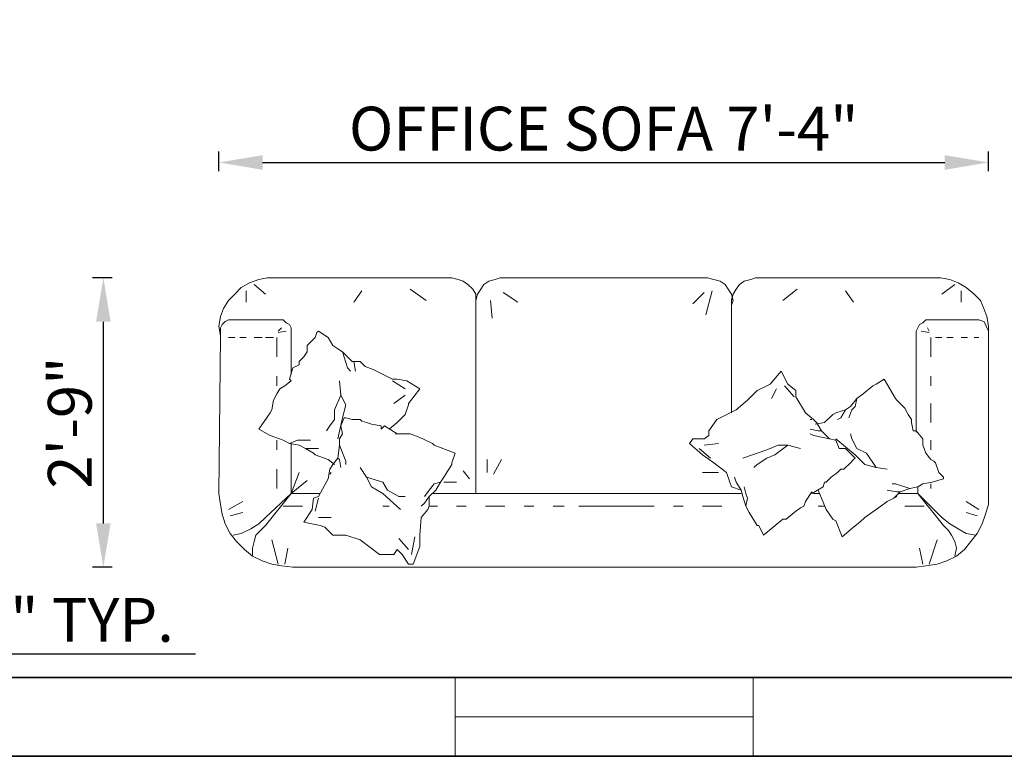
# Model space of a CAD drawing. Units: inches. Extents: x -100 to 766, y -562 to 63.
# Tile 4 of 11: x 268 to 380, y -467 to -383. Entities that reach past the tile are written whole.
import ezdxf

# ---------------------------------------------------------------- set-up
doc = ezdxf.new("R2010")
doc.units = ezdxf.units.IN
for name, color, linetype, lineweight in [('A-ANNO-DIMS', 2, 'Continuous', 18), ('A-GLAZ', 4, 'Continuous', 18), ('A-WALL', 7, 'Continuous', 35), ('furn', 8, 'Continuous', 13)]:
    doc.layers.add(name, color=color, linetype=linetype, lineweight=lineweight)
doc.styles.get("Standard").update_dxf_attribs({"font": 'arial.ttf'})
doc.dimstyles.new('ISO-25', dxfattribs={"dimtxt": 5, "dimasz": 5, "dimexe": 1.25, "dimexo": 0.625, "dimtad": 1, "dimlunit": 3, "dimtxsty": 'Standard', "dimcen": 2.5, "dimadec": 0, "dimazin": 0, "dimtfac": 1, "dimtmove": 0, "dimatfit": 3, "dimfxl": 1, "dimfxlon": 1, "dimarcsym": 0})

# ---------------------------------------------------------------- blocks, each defined once
blk = doc.blocks.new('sofa-36')
at = {"color": 0, "linetype": 'ByBlock'}
for p, q in [((-0.135, 0.885), (-0.105, 0.895)), ((-0.105, 0.895), (-0.135, 0.885)), ((-0.105, 0.895), (-0.08, 0.9)), ((-0.08, 0.9), (-0.105, 0.895)), ((-0.08, 0.9), (0.495, 0.9)), ((0.495, 0.9), (-0.08, 0.9)), ((0.495, 0.9), (0.515, 0.895)), ((0.515, 0.895), (0.495, 0.9)), ((0.515, 0.895), (0.53, 0.89)), ((0.53, 0.89), (0.515, 0.895)), ((0.53, 0.89), (0.545, 0.88)), ((0.545, 0.88), (0.53, 0.89)), ((0.595, 0.88), (0.61, 0.89)), ((0.595, 0.88), (0.61, 0.89)), ((0.61, 0.89), (0.63, 0.895)), ((0.61, 0.89), (0.63, 0.895)), ((0.63, 0.895), (0.645, 0.9)), ((0.63, 0.895), (0.645, 0.9)), ((0.645, 0.9), (0.87, 0.9)), ((0.87, 0.9), (0.645, 0.9)), ((0.87, 0.9), (1.29, 0.9)), ((1.29, 0.9), (0.87, 0.9)), ((1.29, 0.9), (1.31, 0.895)), ((1.31, 0.895), (1.29, 0.9)), ((1.31, 0.895), (1.33, 0.89)), ((1.33, 0.89), (1.31, 0.895)), ((1.33, 0.89), (1.345, 0.88)), ((1.345, 0.88), (1.33, 0.89)), ((1.39, 0.88), (1.405, 0.89)), ((1.39, 0.88), (1.405, 0.89)), ((1.405, 0.89), (1.425, 0.895)), ((1.405, 0.89), (1.425, 0.895)), ((1.425, 0.895), (1.44, 0.9)), ((1.425, 0.895), (1.44, 0.9)), ((1.44, 0.9), (2.015, 0.9)), ((2.015, 0.9), (1.44, 0.9)), ((2.015, 0.9), (2.045, 0.895)), ((2.045, 0.895), (2.015, 0.9)), ((2.045, 0.895), (2.07, 0.885)), ((2.07, 0.885), (2.045, 0.895)), ((-0.18, 0.85), (-0.16, 0.87)), ((-0.16, 0.87), (-0.18, 0.85)), ((-0.16, 0.87), (-0.135, 0.885)), ((-0.135, 0.885), (-0.16, 0.87)), ((-0.145, 0.825), (-0.145, 0.86)), ((-0.085, 0.85), (-0.12, 0.88)), ((0.19, 0.825), (0.215, 0.86)), ((0.415, 0.83), (0.365, 0.865)), ((0.545, 0.88), (0.56, 0.865)), ((0.56, 0.865), (0.545, 0.88)), ((0.56, 0.865), (0.57, 0.85)), ((0.57, 0.85), (0.56, 0.865)), ((0.575, 0.85), (0.585, 0.865)), ((0.575, 0.85), (0.585, 0.865)), ((0.585, 0.865), (0.595, 0.88)), ((0.585, 0.865), (0.595, 0.88)), ((1.305, 0.86), (1.285, 0.785)), ((1.345, 0.88), (1.355, 0.865)), ((1.355, 0.865), (1.345, 0.88)), ((1.355, 0.865), (1.365, 0.85)), ((1.365, 0.85), (1.355, 0.865)), ((1.37, 0.85), (1.38, 0.865)), ((1.37, 0.85), (1.38, 0.865)), ((1.38, 0.865), (1.39, 0.88)), ((1.38, 0.865), (1.39, 0.88)), ((1.525, 0.83), (1.57, 0.865)), ((1.745, 0.825), (1.72, 0.86)), ((2.02, 0.85), (2.06, 0.88)), ((2.07, 0.885), (2.095, 0.87)), ((2.095, 0.87), (2.07, 0.885)), ((2.08, 0.825), (2.08, 0.86)), ((2.095, 0.87), (2.12, 0.85)), ((2.12, 0.85), (2.095, 0.87)), ((-0.215, 0.805), (-0.2, 0.83)), ((-0.2, 0.83), (-0.215, 0.805)), ((-0.2, 0.83), (-0.18, 0.85)), ((-0.18, 0.85), (-0.2, 0.83)), ((0.57, 0.83), (0.575, 0.85)), ((0.57, 0.85), (0.57, 0.83)), ((0.57, 0.83), (0.57, 0.85)), ((0.57, 0.83), (0.575, 0.85)), ((0.57, 0.835), (0.57, 0.23)), ((0.57, 0.815), (0.57, 0.83)), ((0.57, 0.815), (0.57, 0.83)), ((0.615, 0.83), (0.62, 0.775)), ((0.655, 0.855), (0.7, 0.825)), ((1.28, 0.855), (1.245, 0.82)), ((1.365, 0.85), (1.3675, 0.84)), ((1.37, 0.83), (1.365, 0.85)), ((1.365, 0.83), (1.37, 0.85)), ((1.365, 0.835), (1.365, 0.48)), ((1.365, 0.815), (1.37, 0.83)), ((1.365, 0.815), (1.365, 0.83)), ((1.3675, 0.84), (1.37, 0.85)), ((2.12, 0.85), (2.14, 0.83)), ((2.14, 0.83), (2.12, 0.85)), ((2.14, 0.83), (2.15, 0.805)), ((2.15, 0.805), (2.14, 0.83)), ((-0.225, 0.78), (-0.215, 0.805)), ((-0.215, 0.805), (-0.225, 0.78)), ((2.15, 0.805), (2.16, 0.78)), ((2.16, 0.78), (2.15, 0.805)), ((-0.23, 0.75), (-0.225, 0.78)), ((-0.225, 0.78), (-0.23, 0.75)), ((-0.21, 0.765), (-0.2, 0.77)), ((-0.2, 0.77), (-0.19, 0.77)), ((-0.19, 0.77), (-0.175, 0.77)), ((-0.175, 0.77), (-0.055, 0.77)), ((-0.055, 0.77), (-0.04, 0.77)), ((-0.04, 0.77), (-0.03, 0.77)), ((-0.03, 0.77), (-0.02, 0.76)), ((1.96, 0.76), (1.97, 0.77)), ((1.97, 0.77), (1.98, 0.77)), ((1.98, 0.77), (1.99, 0.77)), ((1.99, 0.77), (2.115, 0.77)), ((2.115, 0.77), (2.125, 0.77)), ((2.125, 0.77), (2.135, 0.77)), ((2.135, 0.77), (2.15, 0.765)), ((2.16, 0.78), (2.165, 0.75)), ((2.165, 0.75), (2.16, 0.78)), ((-0.225, 0.72), (-0.23, 0.75)), ((-0.23, 0.75), (-0.225, 0.72)), ((-0.225, 0.745), (-0.22, 0.755)), ((-0.225, 0.735), (-0.225, 0.745)), ((-0.22, 0.755), (-0.21, 0.765)), ((-0.045, 0.735), (-0.035, 0.745)), ((-0.02, 0.76), (-0.01, 0.755)), ((-0.01, 0.755), (-0.005, 0.745)), ((-0.005, 0.745), (-0.005, 0.735)), ((1.94, 0.735), (1.945, 0.745)), ((1.945, 0.745), (1.95, 0.755)), ((1.95, 0.755), (1.96, 0.76)), ((1.98, 0.735), (1.975, 0.745)), ((2.15, 0.765), (2.155, 0.755)), ((2.155, 0.755), (2.16, 0.745)), ((2.16, 0.745), (2.165, 0.735)), ((2.165, 0.75), (2.165, 0.72)), ((2.165, 0.72), (2.165, 0.75)), ((-0.23, 0.23), (-0.225, 0.72)), ((-0.23, 0.23), (-0.225, 0.72)), ((-0.225, 0.72), (-0.225, 0.735)), ((-0.2, 0.715), (-0.18, 0.715)), ((-0.165, 0.715), (-0.145, 0.715)), ((-0.12, 0.715), (-0.095, 0.715)), ((-0.085, 0.715), (-0.06, 0.715)), ((-0.05, 0.715), (-0.05, 0.655)), ((-0.045, 0.73), (-0.02, 0.735)), ((-0.005, 0.735), (-0.005, 0.72)), ((-0.005, 0.72), (-0.005, 0.6)), ((0.07, 0.715), (0.045, 0.69)), ((0.075, 0.73), (0.07, 0.715)), ((0.08, 0.735), (0.075, 0.73)), ((0.11, 0.715), (0.08, 0.735)), ((0.125, 0.69), (0.11, 0.715)), ((1.94, 0.72), (1.94, 0.735)), ((1.94, 0.42), (1.94, 0.72)), ((1.98, 0.73), (1.955, 0.735)), ((1.985, 0.715), (1.985, 0.655)), ((2.02, 0.715), (2, 0.715)), ((2.055, 0.715), (2.035, 0.715)), ((2.1, 0.715), (2.08, 0.715)), ((2.135, 0.715), (2.12, 0.715)), ((2.165, 0.735), (2.165, 0.72)), ((2.165, 0.72), (2.165, 0.23)), ((2.165, 0.72), (2.165, 0.23)), ((0.045, 0.69), (0.045, 0.68)), ((0.045, 0.68), (0.045, 0.67)), ((0.14, 0.68), (0.125, 0.69)), ((0.155, 0.67), (0.14, 0.68)), ((0.035, 0.655), (0.02, 0.64)), ((0.045, 0.67), (0.035, 0.655)), ((0.155, 0.67), (0.17, 0.62)), ((0.185, 0.64), (0.155, 0.67)), ((0, 0.62), (-0.01, 0.585)), ((0.02, 0.63), (0, 0.62)), ((0.02, 0.64), (0.02, 0.63)), ((0.17, 0.62), (0.18, 0.61)), ((0.185, 0.64), (0.21, 0.64)), ((0.19, 0.64), (0.185, 0.64)), ((0.195, 0.61), (0.19, 0.64)), ((0.21, 0.64), (0.225, 0.625)), ((0.225, 0.625), (0.25, 0.615)), ((0.235, 0.62), (0.235, 0.62)), ((0.25, 0.615), (0.31, 0.585)), ((-0.05, 0.595), (-0.05, 0.565)), ((-0.01, 0.585), (-0.005, 0.58)), ((0.31, 0.585), (0.325, 0.585)), ((0.325, 0.585), (0.355, 0.58)), ((1.52, 0.61), (1.485, 0.57)), ((1.54, 0.57), (1.52, 0.61)), ((1.815, 0.57), (1.84, 0.585)), ((1.84, 0.585), (1.875, 0.525)), ((1.985, 0.595), (1.985, 0.565)), ((-0.04, 0.555), (-0.05, 0.54)), ((-0.025, 0.565), (-0.04, 0.555)), ((-0.005, 0.58), (-0.025, 0.565)), ((0.15, 0.535), (0.145, 0.58)), ((0.35, 0.555), (0.31, 0.58)), ((0.355, 0.58), (0.395, 0.555)), ((0.395, 0.555), (0.36, 0.51)), ((1.475, 0.565), (1.445, 0.55)), ((1.485, 0.57), (1.475, 0.565)), ((1.505, 0.555), (1.49, 0.525)), ((1.53, 0.565), (1.56, 0.53)), ((1.565, 0.55), (1.54, 0.57)), ((1.775, 0.54), (1.805, 0.565)), ((1.805, 0.565), (1.815, 0.57)), ((-0.05, 0.54), (-0.06, 0.52)), ((0.15, 0.535), (0.13, 0.49)), ((0.165, 0.505), (0.15, 0.535)), ((0.35, 0.535), (0.315, 0.51)), ((1.445, 0.55), (1.415, 0.52)), ((1.565, 0.53), (1.565, 0.55)), ((1.595, 0.48), (1.565, 0.53)), ((1.735, 0.5), (1.755, 0.525)), ((1.755, 0.525), (1.75, 0.5)), ((1.755, 0.525), (1.775, 0.54)), ((1.875, 0.525), (1.88, 0.52)), ((-0.06, 0.52), (-0.065, 0.49)), ((0.155, 0.465), (0.165, 0.505)), ((0.36, 0.505), (0.35, 0.475)), ((0.36, 0.51), (0.36, 0.505)), ((1.415, 0.52), (1.38, 0.49)), ((1.72, 0.49), (1.735, 0.5)), ((1.75, 0.5), (1.74, 0.49)), ((1.88, 0.52), (1.905, 0.495)), ((1.905, 0.495), (1.915, 0.475)), ((1.985, 0.45), (1.985, 0.51)), ((-0.07, 0.48), (-0.105, 0.43)), ((-0.065, 0.49), (-0.07, 0.48)), ((0.13, 0.46), (0.115, 0.44)), ((0.13, 0.49), (0.13, 0.46)), ((0.14, 0.4), (0.155, 0.465)), ((0.16, 0.465), (0.15, 0.44)), ((0.165, 0.465), (0.16, 0.465)), ((0.185, 0.46), (0.165, 0.465)), ((0.21, 0.46), (0.185, 0.46)), ((0.215, 0.455), (0.21, 0.46)), ((0.35, 0.475), (0.325, 0.45)), ((1.32, 0.46), (1.295, 0.425)), ((1.38, 0.49), (1.32, 0.46)), ((1.62, 0.46), (1.595, 0.48)), ((1.615, 0.46), (1.61, 0.46)), ((1.63, 0.45), (1.62, 0.46)), ((1.68, 0.475), (1.655, 0.45)), ((1.69, 0.48), (1.68, 0.475)), ((1.72, 0.49), (1.69, 0.48)), ((1.695, 0.46), (1.705, 0.465)), ((1.705, 0.465), (1.72, 0.49)), ((1.74, 0.49), (1.73, 0.465)), ((1.915, 0.475), (1.925, 0.46)), ((1.925, 0.46), (1.925, 0.45)), ((-0.105, 0.43), (-0.08, 0.415)), ((0.115, 0.44), (0.105, 0.425)), ((0.15, 0.44), (0.155, 0.415)), ((0.23, 0.45), (0.215, 0.455)), ((0.245, 0.445), (0.23, 0.45)), ((0.275, 0.44), (0.245, 0.445)), ((0.275, 0.43), (0.275, 0.44)), ((0.285, 0.44), (0.275, 0.43)), ((0.325, 0.415), (0.285, 0.44)), ((0.325, 0.45), (0.3, 0.43)), ((1.61, 0.43), (1.635, 0.425)), ((1.655, 0.45), (1.625, 0.445)), ((1.645, 0.425), (1.63, 0.45)), ((1.925, 0.45), (1.93, 0.425)), ((-0.08, 0.415), (-0.07, 0.41)), ((-0.07, 0.41), (-0.03, 0.395)), ((0.155, 0.415), (0.145, 0.4)), ((0.145, 0.4), (0.145, 0.38)), ((0.32, 0.415), (0.325, 0.415)), ((0.355, 0.415), (0.32, 0.415)), ((0.365, 0.415), (0.355, 0.415)), ((0.38, 0.41), (0.365, 0.415)), ((0.405, 0.4), (0.38, 0.41)), ((0.435, 0.385), (0.405, 0.4)), ((1.245, 0.4), (1.235, 0.385)), ((1.28, 0.4), (1.245, 0.4)), ((1.295, 0.41), (1.28, 0.4)), ((1.295, 0.425), (1.295, 0.41)), ((1.62, 0.41), (1.61, 0.415)), ((1.67, 0.4), (1.62, 0.41)), ((1.635, 0.425), (1.645, 0.425)), ((1.645, 0.425), (1.67, 0.4)), ((1.67, 0.4), (1.69, 0.395)), ((1.69, 0.4), (1.75, 0.35)), ((1.74, 0.4), (1.735, 0.415)), ((1.755, 0.37), (1.74, 0.4)), ((1.93, 0.425), (1.94, 0.425)), ((1.94, 0.425), (1.96, 0.4)), ((1.96, 0.4), (1.96, 0.38)), ((-0.05, 0.365), (-0.05, 0.395)), ((-0.03, 0.395), (-0.01, 0.385)), ((-0.01, 0.385), (0.015, 0.395)), ((-0.01, 0.385), (0.02, 0.38)), ((-0.005, 0.385), (-0.005, 0.23)), ((0.015, 0.395), (0.03, 0.395)), ((0.02, 0.38), (0.04, 0.37)), ((0.03, 0.395), (0.055, 0.395)), ((0.04, 0.37), (0.065, 0.355)), ((0.04, 0.37), (0.065, 0.37)), ((0.065, 0.37), (0.08, 0.37)), ((0.145, 0.38), (0.14, 0.34)), ((0.145, 0.38), (0.165, 0.33)), ((0.44, 0.38), (0.435, 0.385)), ((0.505, 0.355), (0.44, 0.38)), ((1.235, 0.385), (1.275, 0.35)), ((1.265, 0.37), (1.3, 0.34)), ((1.28, 0.38), (1.325, 0.385)), ((1.475, 0.365), (1.51, 0.38)), ((1.54, 0.38), (1.5, 0.35)), ((1.51, 0.38), (1.54, 0.38)), ((1.54, 0.38), (1.58, 0.37)), ((1.69, 0.395), (1.7, 0.37)), ((1.7, 0.37), (1.72, 0.37)), ((1.72, 0.37), (1.75, 0.34)), ((1.785, 0.355), (1.755, 0.37)), ((1.96, 0.38), (1.965, 0.37)), ((1.965, 0.37), (1.97, 0.355)), ((1.985, 0.365), (1.985, 0.395)), ((0.065, 0.355), (0.07, 0.35)), ((0.07, 0.35), (0.11, 0.335)), ((0.14, 0.34), (0.125, 0.32)), ((0.14, 0.34), (0.145, 0.335)), ((0.495, 0.325), (0.505, 0.355)), ((1.275, 0.35), (1.31, 0.325)), ((1.4, 0.34), (1.475, 0.365)), ((1.475, 0.34), (1.445, 0.32)), ((1.5, 0.35), (1.475, 0.34)), ((1.75, 0.34), (1.745, 0.335)), ((1.75, 0.35), (1.78, 0.32)), ((1.815, 0.31), (1.785, 0.355)), ((1.97, 0.355), (1.985, 0.335)), ((0.11, 0.335), (0.13, 0.32)), ((0.125, 0.32), (0.115, 0.305)), ((0.145, 0.335), (0.15, 0.31)), ((0.165, 0.33), (0.165, 0.32)), ((0.23, 0.28), (0.21, 0.31)), ((0.47, 0.28), (0.495, 0.32)), ((0.495, 0.32), (0.495, 0.325)), ((0.605, 0.295), (0.605, 0.335)), ((0.625, 0.29), (0.65, 0.335)), ((1.31, 0.325), (1.35, 0.295)), ((1.445, 0.32), (1.435, 0.31)), ((1.735, 0.325), (1.715, 0.305)), ((1.745, 0.335), (1.735, 0.325)), ((1.78, 0.32), (1.815, 0.31)), ((1.815, 0.31), (1.85, 0.305)), ((1.985, 0.335), (1.995, 0.33)), ((1.995, 0.33), (2, 0.325)), ((2, 0.325), (2.01, 0.295)), ((-0.05, 0.245), (-0.05, 0.305)), ((0.02, 0.295), (-0.005, 0.23)), ((0.115, 0.305), (0.11, 0.275)), ((0.12, 0.295), (0.115, 0.29)), ((0.23, 0.28), (0.28, 0.265)), ((0.245, 0.25), (0.23, 0.28)), ((0.46, 0.265), (0.47, 0.28)), ((0.55, 0.275), (0.53, 0.3)), ((1.325, 0.295), (1.275, 0.295)), ((1.35, 0.295), (1.36, 0.265)), ((1.38, 0.265), (1.375, 0.28)), ((1.675, 0.28), (1.66, 0.265)), ((1.695, 0.295), (1.675, 0.28)), ((1.705, 0.305), (1.695, 0.295)), ((1.715, 0.305), (1.705, 0.305)), ((2.01, 0.295), (2.025, 0.28)), ((2.025, 0.28), (2.025, 0.275)), ((0.045, 0.27), (-0.005, 0.23)), ((0.11, 0.275), (0.08, 0.22)), ((0.28, 0.23), (0.245, 0.25)), ((0.28, 0.265), (0.295, 0.24)), ((0.425, 0.24), (0.44, 0.26)), ((0.44, 0.26), (0.46, 0.265)), ((0.445, 0.24), (0.46, 0.265)), ((0.51, 0.265), (0.47, 0.265)), ((1.36, 0.265), (1.365, 0.25)), ((1.365, 0.25), (1.395, 0.24)), ((1.395, 0.24), (1.38, 0.265)), ((1.41, 0.23), (1.405, 0.25)), ((1.65, 0.25), (1.615, 0.23)), ((1.655, 0.265), (1.65, 0.25)), ((1.66, 0.265), (1.655, 0.265)), ((1.875, 0.26), (1.865, 0.26)), ((1.92, 0.245), (1.875, 0.26)), ((1.945, 0.25), (1.92, 0.245)), ((1.96, 0.26), (1.945, 0.25)), ((1.945, 0.25), (1.945, 0.23)), ((1.99, 0.265), (1.96, 0.26)), ((1.985, 0.245), (1.985, 0.26)), ((2.025, 0.275), (1.99, 0.265)), ((-0.225, 0.195), (-0.23, 0.23)), ((-0.225, 0.195), (-0.23, 0.23)), ((-0.005, 0.23), (-0.085, 0.13)), ((-0.005, 0.23), (-0.085, 0.155)), ((0.085, 0.23), (-0.005, 0.23)), ((0.065, 0.215), (0.06, 0.18)), ((0.08, 0.22), (0.065, 0.215)), ((0.07, 0.175), (0.08, 0.215)), ((0.335, 0.18), (0.28, 0.23)), ((0.295, 0.24), (0.33, 0.22)), ((0.33, 0.22), (0.35, 0.22)), ((0.41, 0.22), (0.425, 0.24)), ((0.425, 0.22), (0.41, 0.2)), ((0.425, 0.22), (0.445, 0.24)), ((0.425, 0.19), (0.425, 0.22)), ((0.435, 0.23), (0.87, 0.23)), ((1.395, 0.23), (0.87, 0.23)), ((1.4, 0.22), (1.395, 0.24)), ((1.41, 0.19), (1.4, 0.22)), ((1.415, 0.215), (1.41, 0.23)), ((1.41, 0.19), (1.415, 0.215)), ((1.615, 0.235), (1.595, 0.205)), ((1.615, 0.23), (1.615, 0.235)), ((1.615, 0.23), (1.615, 0.23)), ((1.64, 0.23), (1.62, 0.23)), ((1.645, 0.215), (1.635, 0.24)), ((1.66, 0.18), (1.645, 0.215)), ((1.88, 0.235), (1.85, 0.24)), ((1.87, 0.215), (1.85, 0.205)), ((1.89, 0.235), (1.87, 0.215)), ((1.87, 0.215), (1.88, 0.22)), ((1.89, 0.235), (1.88, 0.235)), ((1.885, 0.23), (1.945, 0.23)), ((1.92, 0.245), (1.89, 0.235)), ((1.945, 0.23), (2.025, 0.13)), ((1.945, 0.23), (2.02, 0.155)), ((2.165, 0.23), (2.165, 0.195)), ((2.165, 0.23), (2.165, 0.195)), ((-0.22, 0.165), (-0.225, 0.195)), ((-0.22, 0.165), (-0.225, 0.195)), ((-0.2, 0.18), (-0.155, 0.205)), ((-0.03, 0.19), (0.03, 0.19)), ((0.28, 0.19), (0.3, 0.19)), ((0.41, 0.2), (0.4, 0.19)), ((0.42, 0.18), (0.425, 0.19)), ((0.45, 0.19), (0.425, 0.19)), ((0.54, 0.19), (0.51, 0.19)), ((0.6, 0.19), (0.66, 0.19)), ((0.72, 0.19), (0.75, 0.19)), ((0.81, 0.19), (0.845, 0.19)), ((1.125, 0.19), (0.89, 0.19)), ((1.215, 0.19), (1.185, 0.19)), ((1.335, 0.19), (1.275, 0.19)), ((1.42, 0.17), (1.41, 0.19)), ((1.58, 0.185), (1.56, 0.17)), ((1.59, 0.19), (1.58, 0.185)), ((1.595, 0.205), (1.59, 0.19)), ((1.655, 0.19), (1.635, 0.19)), ((1.83, 0.19), (1.78, 0.155)), ((1.85, 0.205), (1.83, 0.19)), ((1.845, 0.2), (1.845, 0.2)), ((1.965, 0.19), (1.905, 0.19)), ((2.135, 0.18), (2.095, 0.205)), ((2.165, 0.195), (2.155, 0.165)), ((2.165, 0.195), (2.155, 0.165)), ((-0.21, 0.135), (-0.22, 0.165)), ((-0.21, 0.135), (-0.22, 0.165)), ((-0.155, 0.17), (-0.195, 0.16)), ((-0.085, 0.155), (-0.105, 0.135)), ((0.06, 0.18), (0.035, 0.14)), ((0.08, 0.155), (0.12, 0.155)), ((0.395, 0.1), (0.4, 0.155)), ((0.4, 0.155), (0.42, 0.18)), ((1.445, 0.13), (1.42, 0.17)), ((1.56, 0.17), (1.535, 0.15)), ((1.68, 0.15), (1.66, 0.18)), ((1.78, 0.155), (1.765, 0.14)), ((2.02, 0.155), (2.045, 0.135)), ((2.095, 0.17), (2.13, 0.16)), ((2.155, 0.165), (2.145, 0.135)), ((2.155, 0.165), (2.145, 0.135)), ((-0.195, 0.105), (-0.21, 0.135)), ((-0.195, 0.105), (-0.21, 0.135)), ((-0.105, 0.135), (-0.13, 0.12)), ((-0.085, 0.13), (-0.1, 0.115)), ((0.035, 0.14), (0.085, 0.13)), ((0.085, 0.13), (0.1, 0.125)), ((0.1, 0.125), (0.125, 0.1)), ((1.45, 0.13), (1.445, 0.13)), ((1.465, 0.1), (1.45, 0.13)), ((1.525, 0.15), (1.465, 0.1)), ((1.535, 0.15), (1.525, 0.15)), ((1.69, 0.145), (1.68, 0.15)), ((1.71, 0.095), (1.69, 0.145)), ((1.745, 0.125), (1.71, 0.095)), ((1.765, 0.14), (1.745, 0.125)), ((2.025, 0.13), (2.04, 0.115)), ((2.045, 0.135), (2.07, 0.12)), ((2.145, 0.135), (2.13, 0.105)), ((2.145, 0.135), (2.13, 0.105)), ((-0.175, 0.08), (-0.195, 0.105)), ((-0.175, 0.08), (-0.195, 0.105)), ((-0.16, 0.105), (-0.185, 0.1)), ((-0.13, 0.12), (-0.16, 0.105)), ((-0.115, 0.1), (-0.12, 0.08)), ((-0.1, 0.115), (-0.115, 0.1)), ((0.125, 0.1), (0.165, 0.1)), ((0.165, 0.1), (0.21, 0.085)), ((0.37, 0.04), (0.38, 0.095)), ((0.395, 0.065), (0.395, 0.1)), ((2.04, 0.115), (2.05, 0.1)), ((2.05, 0.1), (2.06, 0.08)), ((2.07, 0.12), (2.095, 0.105)), ((2.095, 0.105), (2.125, 0.1)), ((2.13, 0.105), (2.11, 0.08)), ((2.13, 0.105), (2.11, 0.08)), ((-0.15, 0.055), (-0.175, 0.08)), ((-0.15, 0.055), (-0.175, 0.08)), ((-0.12, 0.08), (-0.125, 0.06)), ((-0.045, 0.01), (-0.065, 0.085)), ((0.21, 0.085), (0.27, 0.04)), ((0.36, 0.055), (0.33, 0.09)), ((0.375, 0.01), (0.395, 0.065)), ((1.98, 0.01), (2.005, 0.085)), ((2.06, 0.08), (2.065, 0.06)), ((2.11, 0.08), (2.09, 0.055)), ((2.11, 0.08), (2.09, 0.055)), ((-0.125, 0.035), (-0.15, 0.055)), ((-0.125, 0.035), (-0.15, 0.055)), ((-0.125, 0.06), (-0.125, 0.035)), ((-0.095, 0.02), (-0.125, 0.035)), ((-0.095, 0.02), (-0.125, 0.035)), ((-0.015, 0.06), (-0.025, 0.01)), ((0.27, 0.04), (0.315, 0.04)), ((0.315, 0.04), (0.325, 0.055)), ((0.325, 0.055), (0.34, 0.04)), ((0.34, 0.04), (0.36, 0.01)), ((1.95, 0.06), (1.96, 0.01)), ((2.065, 0.035), (2.035, 0.02)), ((2.065, 0.035), (2.035, 0.02)), ((2.065, 0.06), (2.06, 0.035)), ((2.09, 0.055), (2.065, 0.035)), ((2.09, 0.055), (2.065, 0.035)), ((-0.065, 0.01), (-0.095, 0.02)), ((-0.065, 0.01), (-0.095, 0.02)), ((-0.035, 0.005), (-0.065, 0.01)), ((-0.035, 0.005), (-0.065, 0.01)), ((0, 0), (-0.035, 0.005)), ((0, 0), (-0.035, 0.005)), ((1.94, 0), (0, 0)), ((1.94, 0), (0, 0)), ((0.36, 0.01), (0.375, 0.01)), ((1.97, 0.005), (1.94, 0)), ((1.97, 0.005), (1.94, 0)), ((2.005, 0.01), (1.97, 0.005)), ((2.005, 0.01), (1.97, 0.005)), ((2.035, 0.02), (2.005, 0.01)), ((2.035, 0.02), (2.005, 0.01))]:
    blk.add_line(p, q, dxfattribs=at)
blk = doc.blocks.new('WIN-34IN')
blk.add_line((4.5, 34), (4.5, 0))
blk.add_lwpolyline([(0, 34), (9, 34), (9, 0), (0, 0)], close=True)
blk = doc.blocks.new('*D22')
at = {"layer": 'A-ANNO-DIMS', "color": 0, "lineweight": -2, "transparency": 16777216}
for p, q in [((193.47, -456.51), (193.47, -454.26)), ((211.47, -456.51), (211.47, -454.26)), ((198.47, -455.51), (206.47, -455.51)), ((211.47, -455.51), (287.98, -455.51))]:
    blk.add_line(p, q, dxfattribs=at)
at = {"layer": 'A-ANNO-DIMS', "color": 0, "transparency": 16777216}
for points in [[(198.47, -454.68), (198.47, -456.35), (193.47, -455.51)], [(206.47, -454.68), (206.47, -456.35), (211.47, -455.51)]]:
    blk.add_solid(points, dxfattribs=at)
at = {"layer": 'Defpoints', "color": 0, "transparency": 16777216}
for p in [(211.47, -455.51), (193.47, -458.21), (211.47, -458.21)]:
    blk.add_point(p, dxfattribs=at)
at = {"layer": 'A-ANNO-DIMS', "color": 0, "transparency": 16777216, "insert": (252.23, -452.3), "char_height": 5, "attachment_point": 5}
blk.add_mtext('WINDOW C 1\'-6" TYP.', dxfattribs=at)
blk = doc.blocks.new('*D34')
at = {"layer": 'A-ANNO-DIMS', "color": 0, "lineweight": -2, "transparency": 16777216}
for p, q in [((290.65, -400.49), (290.65, -398.24)), ((378.46, -400.49), (378.46, -398.24)), ((295.65, -399.49), (373.46, -399.49))]:
    blk.add_line(p, q, dxfattribs=at)
at = {"layer": 'A-ANNO-DIMS', "color": 0, "transparency": 16777216}
for points in [[(295.65, -398.66), (295.65, -400.33), (290.65, -399.49)], [(373.46, -398.66), (373.46, -400.33), (378.46, -399.49)]]:
    blk.add_solid(points, dxfattribs=at)
at = {"layer": 'Defpoints', "color": 0, "transparency": 16777216}
for p in [(378.46, -399.49), (290.65, -412.66), (378.46, -412.66)]:
    blk.add_point(p, dxfattribs=at)
at = {"layer": 'A-ANNO-DIMS', "color": 0, "transparency": 16777216, "insert": (334.56, -396.28), "char_height": 5, "attachment_point": 5}
blk.add_mtext('OFFICE SOFA 7\'-4"', dxfattribs=at)
blk = doc.blocks.new('*D35')
at = {"layer": 'A-ANNO-DIMS', "color": 0, "lineweight": -2, "transparency": 16777216}
for p, q in [((278.48, -412.66), (276.23, -412.66)), ((277.48, -440.66), (277.48, -417.66)), ((278.48, -445.66), (276.23, -445.66))]:
    blk.add_line(p, q, dxfattribs=at)
at = {"layer": 'A-ANNO-DIMS', "color": 0, "transparency": 16777216}
for points in [[(276.65, -417.66), (278.31, -417.66), (277.48, -412.66)], [(276.65, -440.66), (278.31, -440.66), (277.48, -445.66)]]:
    blk.add_solid(points, dxfattribs=at)
at = {"layer": 'Defpoints', "color": 0, "transparency": 16777216}
for p in [(277.48, -412.66), (290.65, -412.66), (290.65, -445.66)]:
    blk.add_point(p, dxfattribs=at)
at = {"layer": 'A-ANNO-DIMS', "color": 0, "transparency": 16777216, "insert": (274.3, -429.16), "char_height": 5, "attachment_point": 5, "rotation": 90}
blk.add_mtext('2\'-9"', dxfattribs=at)
blk = doc.blocks.new('*D49')
at = {"layer": 'A-ANNO-DIMS', "color": 0, "lineweight": -2, "transparency": 16777216}
for p, q in [((-88.51, -356.21), (-90.76, -356.21)), ((-89.51, -361.21), (-89.51, -417.21)), ((-88.51, -422.21), (-90.76, -422.21))]:
    blk.add_line(p, q, dxfattribs=at)
at = {"layer": 'A-ANNO-DIMS', "color": 0, "transparency": 16777216}
for points in [[(-90.35, -361.21), (-88.68, -361.21), (-89.51, -356.21)], [(-90.35, -417.21), (-88.68, -417.21), (-89.51, -422.21)]]:
    blk.add_solid(points, dxfattribs=at)
at = {"layer": 'Defpoints', "color": 0, "transparency": 16777216}
for p in [(562.39, -356.21), (-89.51, -422.21), (562.39, -422.21)]:
    blk.add_point(p, dxfattribs=at)
at = {"layer": 'A-ANNO-DIMS', "color": 0, "transparency": 16777216, "insert": (-92.69, -389.21), "char_height": 5, "attachment_point": 5, "rotation": 90}
blk.add_mtext('5\'-6"', dxfattribs=at)
blk = doc.blocks.new('*D70')
at = {"layer": 'A-ANNO-DIMS', "color": 0, "lineweight": -2, "transparency": 16777216}
for p, q in [((-88.51, -376.85), (-90.76, -376.85)), ((-89.51, -381.85), (-89.51, -419.34)), ((-88.51, -424.34), (-90.76, -424.34))]:
    blk.add_line(p, q, dxfattribs=at)
at = {"layer": 'A-ANNO-DIMS', "color": 0, "transparency": 16777216}
for points in [[(-90.35, -381.85), (-88.68, -381.85), (-89.51, -376.85)], [(-90.35, -419.34), (-88.68, -419.34), (-89.51, -424.34)]]:
    blk.add_solid(points, dxfattribs=at)
at = {"layer": 'Defpoints', "color": 0, "transparency": 16777216}
for p in [(679.5, -376.85), (-89.51, -424.34), (679.5, -424.34)]:
    blk.add_point(p, dxfattribs=at)
at = {"layer": 'A-ANNO-DIMS', "color": 0, "transparency": 16777216, "insert": (-92.73, -400.59), "char_height": 5, "attachment_point": 5, "rotation": 90}
blk.add_mtext('3\'-11 1/2"', dxfattribs=at)
blk = doc.blocks.new('*D73')
at = {"layer": 'A-ANNO-DIMS', "color": 0, "lineweight": -2, "transparency": 16777216}
for p, q in [((-88.51, -345.04), (-90.76, -345.04)), ((-89.51, -350.04), (-89.51, -401.82)), ((-88.51, -406.82), (-90.76, -406.82))]:
    blk.add_line(p, q, dxfattribs=at)
at = {"layer": 'A-ANNO-DIMS', "color": 0, "transparency": 16777216}
for points in [[(-90.35, -350.04), (-88.68, -350.04), (-89.51, -345.04)], [(-90.35, -401.82), (-88.68, -401.82), (-89.51, -406.82)]]:
    blk.add_solid(points, dxfattribs=at)
at = {"layer": 'Defpoints', "color": 0, "transparency": 16777216}
for p in [(475.3, -345.04), (-89.51, -406.82), (475.3, -406.82)]:
    blk.add_point(p, dxfattribs=at)
at = {"layer": 'A-ANNO-DIMS', "color": 0, "transparency": 16777216, "insert": (-92.69, -375.93), "char_height": 5, "attachment_point": 5, "rotation": 90}
blk.add_mtext('5\'-2"', dxfattribs=at)
blk = doc.blocks.new('*D80')
at = {"layer": 'A-ANNO-DIMS', "color": 0, "lineweight": -2, "transparency": 16777216}
for p, q in [((241.52, -558.16), (236.52, -558.16)), ((246.52, -557.16), (246.52, -559.41)), ((246.52, -558.16), (250.39, -558.16)), ((250.39, -557.16), (250.39, -559.41)), ((255.39, -558.16), (274.93, -558.16))]:
    blk.add_line(p, q, dxfattribs=at)
at = {"layer": 'A-ANNO-DIMS', "color": 0, "transparency": 16777216}
for points in [[(241.52, -557.32), (241.52, -558.99), (246.52, -558.16)], [(255.39, -557.32), (255.39, -558.99), (250.39, -558.16)]]:
    blk.add_solid(points, dxfattribs=at)
at = {"layer": 'Defpoints', "color": 0, "transparency": 16777216}
for p in [(246.52, -368.21), (250.39, -368.21), (250.39, -558.16)]:
    blk.add_point(p, dxfattribs=at)
at = {"layer": 'A-ANNO-DIMS', "color": 0, "transparency": 16777216, "insert": (267.66, -554.98), "char_height": 5, "attachment_point": 5}
blk.add_mtext('0\'-4"', dxfattribs=at)
blk = doc.blocks.new('*D83')
at = {"layer": 'A-ANNO-DIMS', "color": 0, "lineweight": -2, "transparency": 16777216}
for p, q in [((-88.51, -422.21), (-90.76, -422.21)), ((-89.51, -427.21), (-89.51, -453.21)), ((-88.51, -458.21), (-90.76, -458.21))]:
    blk.add_line(p, q, dxfattribs=at)
at = {"layer": 'A-ANNO-DIMS', "color": 0, "transparency": 16777216}
for points in [[(-90.35, -427.21), (-88.68, -427.21), (-89.51, -422.21)], [(-90.35, -453.21), (-88.68, -453.21), (-89.51, -458.21)]]:
    blk.add_solid(points, dxfattribs=at)
at = {"layer": 'Defpoints', "color": 0, "transparency": 16777216}
for p in [(562.39, -422.21), (-89.51, -458.21), (562.39, -458.21)]:
    blk.add_point(p, dxfattribs=at)
at = {"layer": 'A-ANNO-DIMS', "color": 0, "transparency": 16777216, "insert": (-92.69, -440.21), "char_height": 5, "attachment_point": 5, "rotation": 90}
blk.add_mtext('3\'-0"', dxfattribs=at)
blk = doc.blocks.new('*D87')
at = {"layer": 'A-ANNO-DIMS', "color": 0, "lineweight": -2, "transparency": 16777216}
for p, q in [((310.41, -557.16), (310.41, -559.41)), ((315.41, -558.16), (352.79, -558.16)), ((357.79, -557.16), (357.79, -559.41))]:
    blk.add_line(p, q, dxfattribs=at)
at = {"layer": 'A-ANNO-DIMS', "color": 0, "transparency": 16777216}
for points in [[(315.41, -557.32), (315.41, -558.99), (310.41, -558.16)], [(352.79, -557.32), (352.79, -558.99), (357.79, -558.16)]]:
    blk.add_solid(points, dxfattribs=at)
at = {"layer": 'Defpoints', "color": 0, "transparency": 16777216}
for p in [(310.41, -121.91), (357.79, -121.91), (357.79, -558.16)]:
    blk.add_point(p, dxfattribs=at)
at = {"layer": 'A-ANNO-DIMS', "color": 0, "transparency": 16777216, "insert": (334.1, -554.94), "char_height": 5, "attachment_point": 5}
blk.add_mtext('3\'-11 1/2"', dxfattribs=at)

msp = doc.modelspace()

# ---------------------------------------------------------------- linework, layer by layer
at = {"layer": 'A-WALL'}
msp.add_line((532.388, -458.214), (250.388, -458.214), dxfattribs=at)
msp.add_lwpolyline([(1.388, 12.786), (721.388, 12.786), (721.388, -467.214), (1.388, -467.214)], close=True, dxfattribs=at)

# ---------------------------------------------------------------- block references
at = {"layer": 'A-GLAZ', "rotation": 270.0000000000002}
msp.add_blockref('WIN-34IN', (317.595, -458.215), dxfattribs=at)
at = {"layer": 'furn', "xscale": 36.66436083614781, "yscale": 36.66436083614781, "zscale": 36.66436083614781}
msp.add_blockref('sofa-36', (299.084, -445.662), dxfattribs=at)

# ---------------------------------------------------------------- dimensions: what is measured, and where the dimension line sits
at = {"layer": 'A-ANNO-DIMS'}
for base, p1, p2, picture, middle in [((357.792, -558.156), (310.414, -121.911), (357.792, -121.911), '*D87', (334.103, -554.944)), ((250.388, -558.156), (246.522, -368.214), (250.388, -368.214), '*D80', (267.658, -554.979))]:
    dim = msp.add_linear_dim(base=base, p1=p1, p2=p2, dimstyle='ISO-25', override={"dimdec": 1, "dimlfac": 1, "dimrnd": 0, "dimzin": 1, "dimdsep": 46, "dimlunit": 4, "dimfrac": 2}, dxfattribs=at)
    dim.commit()
    dim.dimension.update_dxf_attribs({"geometry": picture, "text_midpoint": middle})
for base, p1, p2, picture, middle in [((-89.513, -406.822), (475.3, -345.045), (475.3, -406.822), '*D73', (-92.691, -375.933)), ((-89.513, -422.214), (562.394, -356.214), (562.394, -422.214), '*D49', (-92.691, -389.214)), ((-89.513, -424.336), (679.495, -376.848), (679.495, -424.336), '*D70', (-92.725, -400.592)), ((277.48, -412.664), (290.652, -445.662), (290.652, -412.664), '*D35', (274.302, -429.163)), ((-89.513, -458.214), (562.394, -422.214), (562.394, -458.214), '*D83', (-92.693, -440.214))]:
    dim = msp.add_linear_dim(base=base, p1=p1, p2=p2, angle=90, dimstyle='ISO-25', override={"dimdec": 1, "dimlfac": 1, "dimrnd": 0, "dimzin": 1, "dimdsep": 46, "dimlunit": 4, "dimfrac": 2}, dxfattribs=at)
    dim.commit()
    dim.dimension.update_dxf_attribs({"geometry": picture, "text_midpoint": middle})
dim = msp.add_linear_dim(base=(378.463, -399.492), p1=(290.652, -412.664), p2=(378.463, -412.664), text='OFFICE SOFA <>', dimstyle='ISO-25', override={"dimdec": 1, "dimlfac": 1, "dimrnd": 0, "dimzin": 1, "dimdsep": 46, "dimlunit": 4, "dimfrac": 2}, dxfattribs=at)
dim.commit()
dim.dimension.update_dxf_attribs({"geometry": '*D34', "text_midpoint": (334.557, -396.28)})
dim = msp.add_linear_dim(base=(211.473, -455.514), p1=(193.473, -458.214), p2=(211.473, -458.214), angle=0, text='WINDOW C <> TYP.', dimstyle='ISO-25', override={"dimdec": 1, "dimlfac": 1, "dimrnd": 0, "dimzin": 1, "dimdsep": 46, "dimlunit": 4, "dimfrac": 2}, dxfattribs=at)
dim.commit()
dim.dimension.update_dxf_attribs({"geometry": '*D22', "text_midpoint": (252.226, -452.302)})

doc.saveas('drawing.dxf')
